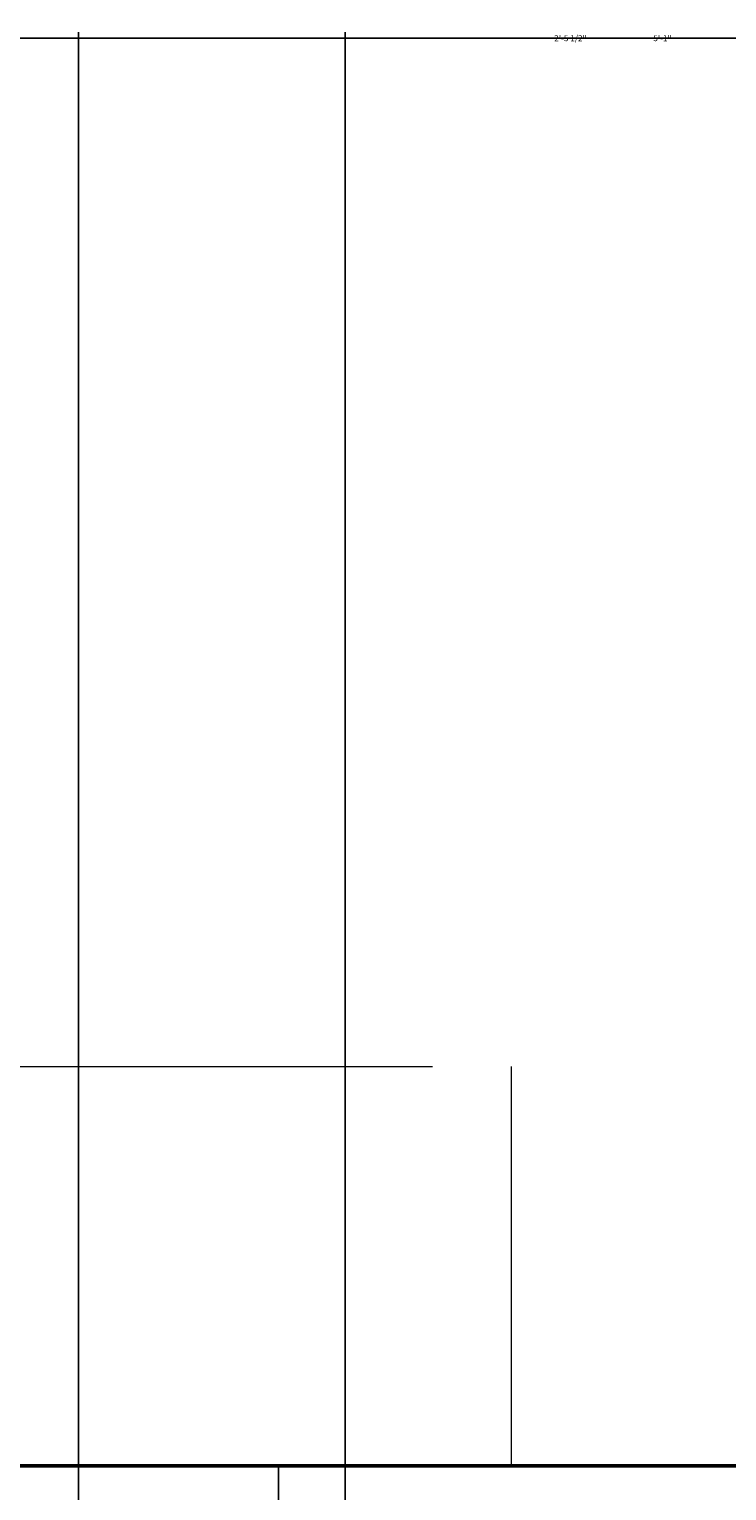
# Model space of a CAD drawing. Units: inches. Extents: x 37 to 824, y -700 to 234.
# Tile 75 of 77: x 370 to 391, y 190 to 234. Entities that reach past the tile are written whole.
import ezdxf

# ---------------------------------------------------------------- set-up
doc = ezdxf.new("R2010")
doc.units = ezdxf.units.IN
doc.header["$MEASUREMENT"] = 0
doc.linetypes.add('DASHED', pattern=[19.05, 12.7, -6.35])
for name, color, linetype, lineweight in [('A-ANNO-DIMS', 2, 'Continuous', 18), ('A-GLAZ', 4, 'Continuous', 25), ('A-ROOF-OVHD', 1, 'DASHED', 18), ('A-WALL', 2, 'Continuous', 50)]:
    doc.layers.add(name, color=color, linetype=linetype, lineweight=lineweight)
doc.styles.get("Standard").update_dxf_attribs({"font": 'arial.ttf'})
doc.dimstyles.get("Standard").update_dxf_attribs({"dimtxt": 0.18, "dimasz": 0.18, "dimexe": 0.18, "dimexo": 0.0625, "dimgap": 0.09, "dimtad": 0, "dimtih": 1, "dimtoh": 1, "dimdec": 1, "dimzin": 0, "dimdsep": 46, "dimlunit": 4, "dimtxsty": 'Standard', "dimcen": 0.09, "dimadec": 0, "dimazin": 0, "dimtfac": 1, "dimtdec": 1, "dimtofl": 0, "dimtmove": 0, "dimatfit": 3, "dimfxl": 1, "dimtolj": 1, "dimtzin": 0, "dimarcsym": 0})

# ---------------------------------------------------------------- blocks, each defined once
blk = doc.blocks.new('WIN-900')
for p, q in [((0, 9), (0, 0)), ((2, 9), (2, 0)), ((20, 9), (20, 0)), ((38, 9), (38, 0)), ((40, 9), (40, 0)), ((38, 5.5), (2, 5.5)), ((38, 3.5), (2, 3.5))]:
    blk.add_line(p, q)
blk = doc.blocks.new('*D47')
at = {"layer": 'A-ANNO-DIMS', "color": 0, "lineweight": -2, "ltscale": 0.5, "transparency": 16777216}
for p, q in [((339.077, 191.153), (339.077, 234.17)), ((379.077, 191.153), (379.077, 234.17)), ((339.257, 233.99), (358.748, 233.99)), ((378.897, 233.99), (359.406, 233.99))]:
    blk.add_line(p, q, dxfattribs=at)
at = {"layer": 'A-ANNO-DIMS', "color": 0, "ltscale": 0.5, "transparency": 16777216}
for points in [[(339.257, 234.02), (339.257, 233.96), (339.077, 233.99)], [(378.897, 234.02), (378.897, 233.96), (379.077, 233.99)]]:
    blk.add_solid(points, dxfattribs=at)
at = {"layer": 'Defpoints', "color": 0, "ltscale": 0.5, "transparency": 16777216}
for p in [(379.077, 233.99), (339.077, 191.09), (379.077, 191.09)]:
    blk.add_point(p, dxfattribs=at)
at = {"layer": 'A-ANNO-DIMS', "color": 0, "ltscale": 0.5, "transparency": 16777216, "insert": (359.077, 233.99), "char_height": 0.18, "attachment_point": 5}
blk.add_mtext('\\A1;3\'-4"', dxfattribs=at)
blk = doc.blocks.new('*D48')
at = {"layer": 'A-ANNO-DIMS', "color": 0, "lineweight": -2, "ltscale": 0.5, "transparency": 16777216}
for p, q in [((379.077, 191.153), (379.077, 234.17)), ((428.077, 191.153), (428.077, 234.17)), ((379.257, 233.99), (403.244, 233.99)), ((427.897, 233.99), (403.91, 233.99))]:
    blk.add_line(p, q, dxfattribs=at)
at = {"layer": 'A-ANNO-DIMS', "color": 0, "ltscale": 0.5, "transparency": 16777216}
for points in [[(379.257, 234.02), (379.257, 233.96), (379.077, 233.99)], [(427.897, 234.02), (427.897, 233.96), (428.077, 233.99)]]:
    blk.add_solid(points, dxfattribs=at)
at = {"layer": 'Defpoints', "color": 0, "ltscale": 0.5, "transparency": 16777216}
for p in [(428.077, 233.99), (379.077, 191.09), (428.077, 191.09)]:
    blk.add_point(p, dxfattribs=at)
at = {"layer": 'A-ANNO-DIMS', "color": 0, "ltscale": 0.5, "transparency": 16777216, "insert": (403.577, 233.99), "char_height": 0.18, "attachment_point": 5}
blk.add_mtext('\\A1;4\'-1"', dxfattribs=at)
blk = doc.blocks.new('*D63')
at = {"layer": 'A-ANNO-DIMS', "color": 0, "lineweight": -2, "ltscale": 0.5, "transparency": 16777216}
for p, q in [((161.077, 191.153), (161.077, 234.17)), ((428.077, 191.153), (428.077, 234.17)), ((161.257, 233.99), (294.176, 233.99)), ((427.897, 233.99), (294.978, 233.99))]:
    blk.add_line(p, q, dxfattribs=at)
at = {"layer": 'A-ANNO-DIMS', "color": 0, "ltscale": 0.5, "transparency": 16777216}
for points in [[(161.257, 234.02), (161.257, 233.96), (161.077, 233.99)], [(427.897, 234.02), (427.897, 233.96), (428.077, 233.99)]]:
    blk.add_solid(points, dxfattribs=at)
at = {"layer": 'Defpoints', "color": 0, "ltscale": 0.5, "transparency": 16777216}
for p in [(428.077, 233.99), (161.077, 191.09), (428.077, 191.09)]:
    blk.add_point(p, dxfattribs=at)
at = {"layer": 'A-ANNO-DIMS', "color": 0, "ltscale": 0.5, "transparency": 16777216, "insert": (294.577, 233.99), "char_height": 0.18, "attachment_point": 5}
blk.add_mtext('\\A1;22\'-3"', dxfattribs=at)
blk = doc.blocks.new('*D74')
at = {"layer": 'A-ANNO-DIMS', "color": 0, "lineweight": -2, "ltscale": 0.5, "transparency": 16777216}
for p, q in [((371.077, 84.153), (371.077, 234.17)), ((400.605, 84.153), (400.605, 234.17)), ((371.257, 233.99), (385.3, 233.99)), ((400.425, 233.99), (386.381, 233.99))]:
    blk.add_line(p, q, dxfattribs=at)
at = {"layer": 'A-ANNO-DIMS', "color": 0, "ltscale": 0.5, "transparency": 16777216}
for points in [[(371.257, 234.02), (371.257, 233.96), (371.077, 233.99)], [(400.425, 234.02), (400.425, 233.96), (400.605, 233.99)]]:
    blk.add_solid(points, dxfattribs=at)
at = {"layer": 'Defpoints', "color": 0, "ltscale": 0.5, "transparency": 16777216}
for p in [(400.605, 233.99), (371.077, 84.09), (400.605, 84.09)]:
    blk.add_point(p, dxfattribs=at)
at = {"layer": 'A-ANNO-DIMS', "color": 0, "ltscale": 0.5, "transparency": 16777216, "insert": (385.841, 233.99), "char_height": 0.18, "attachment_point": 5}
blk.add_mtext('\\A1;2\'-5 1/2"', dxfattribs=at)
blk = doc.blocks.new('*D83')
at = {"layer": 'A-ANNO-DIMS', "color": 0, "lineweight": -2, "ltscale": 0.5, "transparency": 16777216}
for p, q in [((358.132, -206.847), (358.132, 234.17)), ((419.077, -206.847), (419.077, 234.17)), ((358.312, 233.99), (388.275, 233.99)), ((418.897, 233.99), (388.934, 233.99))]:
    blk.add_line(p, q, dxfattribs=at)
at = {"layer": 'A-ANNO-DIMS', "color": 0, "ltscale": 0.5, "transparency": 16777216}
for points in [[(358.312, 234.02), (358.312, 233.96), (358.132, 233.99)], [(418.897, 234.02), (418.897, 233.96), (419.077, 233.99)]]:
    blk.add_solid(points, dxfattribs=at)
at = {"layer": 'Defpoints', "color": 0, "ltscale": 0.5, "transparency": 16777216}
for p in [(419.077, 233.99), (358.132, -206.91), (419.077, -206.91)]:
    blk.add_point(p, dxfattribs=at)
at = {"layer": 'A-ANNO-DIMS', "color": 0, "ltscale": 0.5, "transparency": 16777216, "insert": (388.605, 233.99), "char_height": 0.18, "attachment_point": 5}
blk.add_mtext('\\A1;5\'-1"', dxfattribs=at)

msp = doc.modelspace()

# ---------------------------------------------------------------- linework, layer by layer
at = {"layer": 'A-ROOF-OVHD', "ltscale": 1.5}
for p, q in [((334.077, 203.09), (384.077, 203.09)), ((384.077, 191.09), (384.077, 203.09)), ((379.077, 191.09), (384.077, 191.09))]:
    msp.add_line(p, q, dxfattribs=at)
at = {"layer": 'A-WALL'}
msp.add_line((299.077, 191.09), (428.077, 191.09), dxfattribs=at)

# ---------------------------------------------------------------- block references
at = {"layer": 'A-GLAZ'}
msp.add_blockref('WIN-900', (339.077, 182.09), dxfattribs=at)

# ---------------------------------------------------------------- dimensions: what is measured, and where the dimension line sits
at = {"layer": 'A-ANNO-DIMS', "ltscale": 0.5}
for base, p1, p2, picture, middle in [((428.077, 233.99), (161.077, 191.09), (428.077, 191.09), '*D63', (294.577, 233.99)), ((379.077, 233.99), (339.077, 191.09), (379.077, 191.09), '*D47', (359.077, 233.99)), ((419.077, 233.99), (358.132, -206.91), (419.077, -206.91), '*D83', (388.605, 233.99)), ((400.605, 233.99), (371.077, 84.09), (400.605, 84.09), '*D74', (385.841, 233.99)), ((428.077, 233.99), (379.077, 191.09), (428.077, 191.09), '*D48', (403.577, 233.99))]:
    dim = msp.add_linear_dim(base=base, p1=p1, p2=p2, dimstyle='Standard', override={"dimdec": 1, "dimlfac": 1, "dimrnd": 0, "dimzin": 1, "dimdsep": 46, "dimlunit": 4, "dimfrac": 2}, dxfattribs=at)
    dim.commit()
    dim.dimension.update_dxf_attribs({"geometry": picture, "text_midpoint": middle})

doc.saveas('drawing.dxf')
